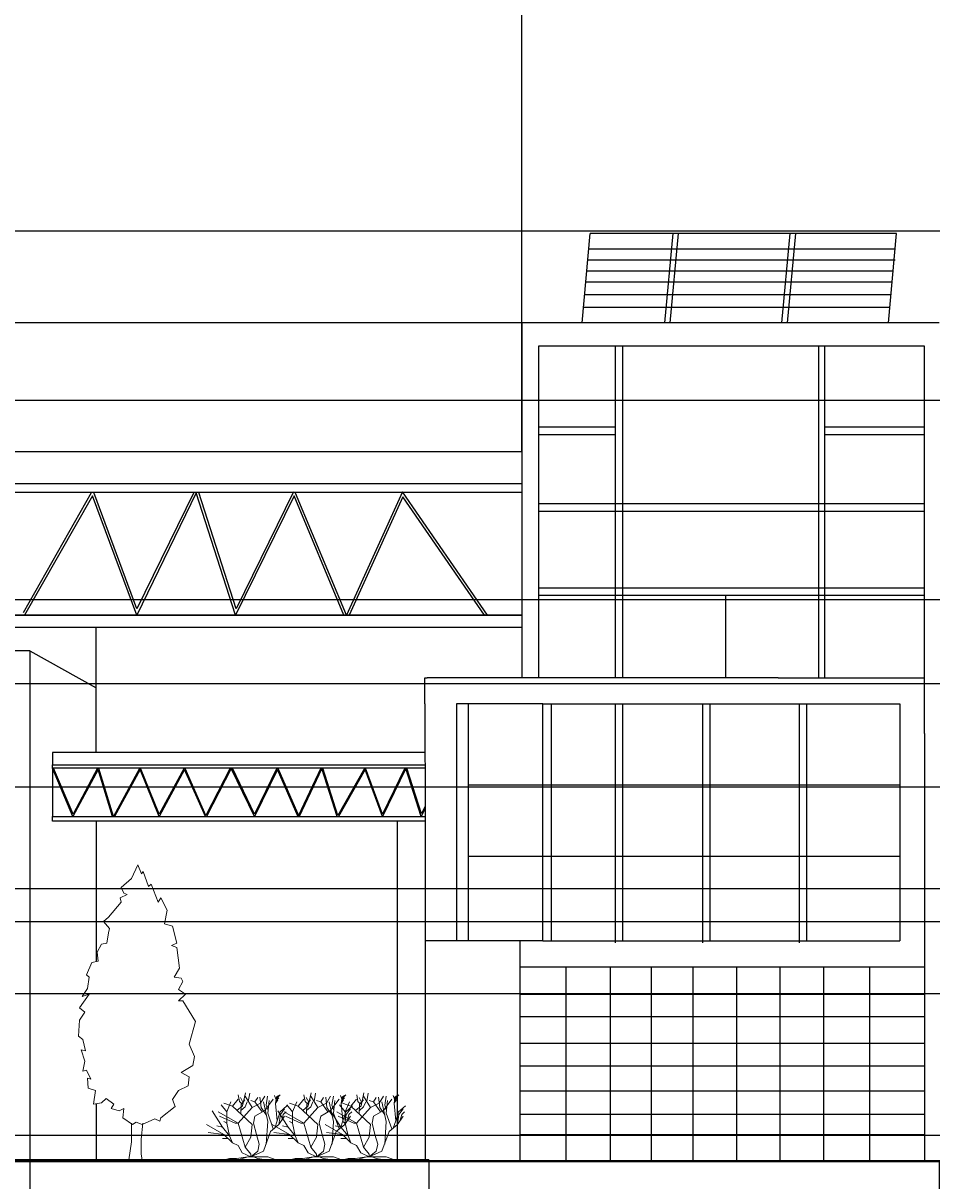
# Model space of a CAD drawing. Units: inches. Extents: x -32109 to 33221, y -19197 to 7608.
# Tile 11 of 25: x -9406 to -5707, y -2204 to 2510. Entities that reach past the tile are written whole.
import ezdxf

# ---------------------------------------------------------------- set-up
doc = ezdxf.new("R2010")
doc.units = ezdxf.units.IN
doc.header["$MEASUREMENT"] = 0
for name, color, linetype, lineweight in [('A-ANNO-DIMS', 2, 'Continuous', 18), ('A-ELEV', 7, 'Continuous', 25), ('L-PLNT', 3, 'Continuous', 13)]:
    doc.layers.add(name, color=color, linetype=linetype, lineweight=lineweight)
doc.styles.get("Standard").update_dxf_attribs({"font": 'arial.ttf'})
doc.dimstyles.get("Standard").update_dxf_attribs({"dimtxt": 0.18, "dimasz": 0.18, "dimexe": 0.18, "dimexo": 0.0625, "dimgap": 0.09, "dimtad": 0, "dimtih": 1, "dimtoh": 1, "dimdec": 4, "dimzin": 0, "dimdsep": 46, "dimtxsty": 'Standard', "dimcen": 0.09, "dimadec": 0, "dimazin": 0, "dimtfac": 1, "dimtdec": 4, "dimtofl": 0, "dimtmove": 0, "dimatfit": 3, "dimfxl": 1, "dimtolj": 1, "dimtzin": 0, "dimarcsym": 0})

# ---------------------------------------------------------------- blocks, each defined once
blk = doc.blocks.new('*U2')
blk.add_lwpolyline([(-2.754, 191.699), (-6.78, 182.851), (-13.682, 176.953), (-11.956, 173.266), (-9.656, 172.529), (-14.257, 170.317), (-13.682, 167.368), (-21.733, 157.783), (-25.184, 154.834), (-21.158, 150.41), (-21.733, 147.461), (-22.884, 140.825), (-26.334, 140.087), (-29.21, 134.926), (-28.635, 129.028), (-32.661, 128.291), (-36.111, 120.18), (-34.386, 118.706), (-35.536, 111.333), (-38.987, 106.171), (-34.386, 107.646), (-40.712, 98.798), (-37.261, 95.849), (-40.712, 90.688), (-41.287, 80.366), (-38.412, 78.154), (-36.686, 70.781), (-39.562, 71.518), (-37.261, 64.145), (-38.412, 57.509), (-36.111, 58.247), (-33.236, 52.348), (-35.536, 53.086), (-34.961, 46.45), (-30.36, 44.975), (-31.51, 36.128), (-26.334, 36.865), (-23.459, 39.814), (-18.283, 36.128), (-20.008, 33.178), (-14.832, 31.704), (-11.956, 33.178), (-12.531, 27.28), (-6.205, 22.856), (-3.905, 24.331), (0.121, 22.856), (8.173, 26.543), (11.624, 25.068), (12.199, 27.28), (21.4, 34.653), (19.675, 39.077), (23.701, 44.975), (30.027, 47.924), (30.602, 53.823), (25.426, 56.772), (32.903, 61.196), (34.053, 67.094), (30.602, 75.205), (34.628, 89.951), (26.576, 103.222), (23.701, 103.222), (28.302, 107.646), (23.701, 110.595), (26.576, 115.756), (25.426, 117.968), (20.825, 118.706), (24.276, 124.604), (22.551, 137.876), (19.1, 139.35), (22.551, 140.825), (19.675, 151.884), (14.499, 153.359), (16.224, 162.207), (12.199, 170.317), (10.473, 167.368), (5.872, 179.165), (4.147, 177.69), (0.696, 187.275), (-0.454, 185.8)], close=True)
for points in [[(-6.813, 23.669), (-6.813, 11.669), (-8.627, 0)], [(0.387, 23.669), (-0.576, 13.271), (-0.576, 3.686), (0, 0)]]:
    blk.add_lwpolyline(points)
blk = doc.blocks.new('*U3')
for p, q in [((-16.8, 16.32), (-15.36, 19.68)), ((-14.88, 18.24), (-12.96, 20.64)), ((-12.471, 19.775), (-12.898, 22.044)), ((-11.677, 19.071), (-12.471, 19.775)), ((-11.28, 19.619), (-12.104, 21.184)), ((-11.921, 18.836), (-10.64, 20.401)), ((-11.433, 18.289), (-10.457, 22.749)), ((-10.579, 18.054), (-9.846, 19.697)), ((-8.16, 17.76), (-10.56, 21.6)), ((-9.48, 19.775), (-8.992, 22.592)), ((-7.2, 19.68), (-8.64, 20.16)), ((-7.2, 19.68), (-6.24, 21.12)), ((-4.8, 16.32), (-7.2, 19.68)), ((-5.086, 17.741), (-5.513, 21.34)), ((-5.28, 19.2), (-3.84, 21.6)), ((-2.88, 12.96), (-4.32, 19.68)), ((-3.84, 16.8), (-0.96, 20.64)), ((-3.377, 18.602), (-2.888, 21.575)), ((-2.88, 15.84), (-2.4, 20.16)), ((-0.508, 21.888), (-0.081, 20.558)), ((-0.203, 19.149), (0.102, 21.34)), ((-0.142, 19.384), (0.59, 20.401)), ((-0.02, 20.01), (0.896, 21.105)), ((0.041, 20.714), (1.384, 22.044)), ((0.102, 21.34), (0.835, 21.888)), ((-18.24, 11.04), (-21.755, 16.655)), ((-12.96, 12.48), (-19.68, 16.32)), ((-16.8, 16.32), (-18.72, 18.72)), ((-14.88, 18.24), (-17.76, 19.2)), ((-16.8, 12.48), (-16.8, 16.32)), ((-8.16, 12), (-14.88, 18.24)), ((-13.325, 16.724), (-11.433, 18.289)), ((-12.96, 12.48), (-8.16, 17.76)), ((-12.043, 15.628), (-11.921, 18.836)), ((-11.982, 16.802), (-10.579, 18.054)), ((-8.16, 17.76), (-5.28, 19.2)), ((-7.2, 14.88), (-3.84, 16.8)), ((-3.377, 15.315), (-5.086, 17.819)), ((-2.766, 16.802), (-3.377, 18.602)), ((-0.96, 10.56), (-2.88, 15.84)), ((0.346, 13.203), (-0.203, 19.149)), ((0.346, 13.203), (1.323, 16.254)), ((1.323, 16.254), (3.642, 18.289)), ((1.44, 15.36), (2.88, 17.28)), ((2.4, 15.36), (3.36, 16.32)), ((-17.76, 8.64), (-23.663, 11.961)), ((-13.92, 12.48), (-19.2, 14.88)), ((-16.8, 12.48), (-17.76, 12.96)), ((-15.84, 8.16), (-16.8, 12.48)), ((-12.96, 12.48), (-13.92, 12.48)), ((-10.56, 4.32), (-12.96, 12.48)), ((-8.64, 7.68), (-8.16, 12)), ((-7.68, 12.48), (-7.2, 14.88)), ((-6.72, 8.64), (-7.68, 12.48)), ((-3.36, 5.28), (-2.88, 12.96)), ((-1.92, 9.6), (0.96, 12)), ((-0.48, 10.8), (0.346, 13.203)), ((0.96, 12), (1.44, 15.36)), ((0.96, 12), (2.88, 14.88)), ((1.92, 13.44), (2.4, 15.36)), ((-17.76, 8.64), (-23.128, 9.222)), ((-18.24, 11.04), (-20.16, 11.52)), ((-15.84, 8.16), (-18.24, 11.04)), ((-14.88, 5.76), (-17.76, 8.64)), ((-14.88, 5.76), (-15.84, 8.16)), ((-5.76, 5.28), (-6.72, 8.64)), ((-4.32, 2.88), (-1.92, 9.6)), ((-16.32, 7.2), (-18.24, 7.2)), ((-12.96, 4.8), (-14.88, 5.76)), ((-11.52, 2.4), (-12.96, 4.8)), ((-10.56, 4.32), (-8.64, 7.68)), ((-8.64, 1.92), (-10.56, 4.32)), ((-6.24, 2.88), (-5.76, 5.28)), ((-15.84, 0.48), (-17.76, 0)), ((-13.44, 0.48), (-15.84, 0.48)), ((-9.6, 0.96), (-13.44, 0.48)), ((-9.6, 0.96), (-12.96, 0)), ((-8.64, 0.96), (-11.52, 2.4)), ((-9.6, 0.96), (-7.68, 0.96)), ((-8.64, 0.96), (-4.32, 2.88)), ((-8.64, 0.96), (-6.24, 2.88)), ((-8.64, 0.96), (-8.64, 1.92)), ((-8.64, 0.96), (-2.88, 0.96)), ((-7.68, 0.96), (-6.24, 0.48)), ((-6.24, 0.48), (-3.36, 0)), ((-2.88, 0.96), (0, 0))]:
    blk.add_line(p, q)
blk = doc.blocks.new('*D10')
at = {"layer": 'A-ANNO-DIMS', "color": 0, "lineweight": -2, "transparency": 16777216}
for p, q in [((-18512.6, -110.2), (-18512.6, 5772)), ((-18512.5, 5771.8), (-202.1, 5771.8)), ((18109.1, 5771.8), (-201.2, 5771.8)), ((18109.3, -101.5), (18109.3, 5772))]:
    blk.add_line(p, q, dxfattribs=at)
at = {"layer": 'A-ANNO-DIMS', "color": 0, "transparency": 16777216}
for points in [[(-18512.5, 5771.9), (-18512.5, 5771.8), (-18512.6, 5771.8)], [(18109.1, 5771.9), (18109.1, 5771.8), (18109.3, 5771.8)]]:
    blk.add_solid(points, dxfattribs=at)
at = {"layer": 'Defpoints', "color": 0, "transparency": 16777216}
for p in [(18109.3, 5771.8), (-18512.6, -110.2), (18109.3, -101.6)]:
    blk.add_point(p, dxfattribs=at)
at = {"layer": 'A-ANNO-DIMS', "color": 0, "transparency": 16777216, "insert": (-201.7, 5771.8), "char_height": 0.18, "attachment_point": 5}
blk.add_mtext('\\A1;36622', dxfattribs=at)
blk = doc.blocks.new('*D11')
at = {"layer": 'A-ANNO-DIMS', "color": 0, "lineweight": -2, "transparency": 16777216}
for p, q in [((14509.6, 1705.2), (25710.6, 1705.2)), ((25710.5, 1705), (25710.5, -209.6)), ((25710.5, -2124.6), (25710.5, -210)), ((-18512.6, -2124.8), (25710.6, -2124.8))]:
    blk.add_line(p, q, dxfattribs=at)
at = {"layer": 'A-ANNO-DIMS', "color": 0, "transparency": 16777216}
for points in [[(25710.4, 1705), (25710.5, 1705), (25710.5, 1705.2)], [(25710.4, -2124.6), (25710.5, -2124.6), (25710.5, -2124.8)]]:
    blk.add_solid(points, dxfattribs=at)
at = {"layer": 'Defpoints', "color": 0, "transparency": 16777216}
for p in [(14509.6, 1705.2), (-18512.6, -2124.8), (25710.5, -2124.8)]:
    blk.add_point(p, dxfattribs=at)
at = {"layer": 'A-ANNO-DIMS', "color": 0, "transparency": 16777216, "insert": (25710.5, -209.8), "char_height": 0.18, "attachment_point": 5}
blk.add_mtext('\\A1;3830', dxfattribs=at)
blk = doc.blocks.new('*D21')
at = {"layer": 'A-ANNO-DIMS', "color": 0, "lineweight": -2, "transparency": 16777216}
for p, q in [((-5532.2, -1149.2), (-24362, -1149.2)), ((-24361.8, -1149.4), (-24361.8, -1636.8)), ((-24361.8, -2124.6), (-24361.8, -1637.2)), ((-5677.1, -2124.8), (-24362, -2124.8))]:
    blk.add_line(p, q, dxfattribs=at)
at = {"layer": 'A-ANNO-DIMS', "color": 0, "transparency": 16777216}
for points in [[(-24361.8, -1149.4), (-24361.8, -1149.4), (-24361.8, -1149.2)], [(-24361.8, -2124.6), (-24361.8, -2124.6), (-24361.8, -2124.8)]]:
    blk.add_solid(points, dxfattribs=at)
at = {"layer": 'Defpoints', "color": 0, "transparency": 16777216}
for p in [(-24361.8, -1149.2), (-5532.1, -1149.2), (-5677.1, -2124.8)]:
    blk.add_point(p, dxfattribs=at)
at = {"layer": 'A-ANNO-DIMS', "color": 0, "transparency": 16777216, "insert": (-24361.8, -1637), "char_height": 0.18, "attachment_point": 5}
blk.add_mtext('\\A1;975.6', dxfattribs=at)
blk = doc.blocks.new('*D27')
at = {"layer": 'A-ANNO-DIMS', "color": 0, "lineweight": -2, "transparency": 16777216}
for p, q in [((-11787, -2124.9), (-11787, -5429.7)), ((-9378.4, -2124.9), (-9378.4, -5429.7)), ((-11786.8, -5429.6), (-10583.2, -5429.6)), ((-9378.6, -5429.6), (-10582.2, -5429.6))]:
    blk.add_line(p, q, dxfattribs=at)
at = {"layer": 'A-ANNO-DIMS', "color": 0, "transparency": 16777216}
for points in [[(-11786.8, -5429.5), (-11786.8, -5429.6), (-11787, -5429.6)], [(-9378.6, -5429.5), (-9378.6, -5429.6), (-9378.4, -5429.6)]]:
    blk.add_solid(points, dxfattribs=at)
at = {"layer": 'Defpoints', "color": 0, "transparency": 16777216}
for p in [(-11787, -2124.8), (-9378.4, -2124.8), (-9378.4, -5429.6)]:
    blk.add_point(p, dxfattribs=at)
at = {"layer": 'A-ANNO-DIMS', "color": 0, "transparency": 16777216, "insert": (-10582.7, -5429.6), "char_height": 0.18, "attachment_point": 5}
blk.add_mtext('\\A1;2408.6', dxfattribs=at)
blk = doc.blocks.new('*D28')
at = {"layer": 'A-ANNO-DIMS', "color": 0, "lineweight": -2, "transparency": 16777216}
for p, q in [((-7754.4, -2118.5), (-7754.4, -5429.7)), ((-9378.4, -2124.9), (-9378.4, -5429.7)), ((-9378.2, -5429.6), (-8566.7, -5429.6)), ((-7754.6, -5429.6), (-8566, -5429.6))]:
    blk.add_line(p, q, dxfattribs=at)
at = {"layer": 'A-ANNO-DIMS', "color": 0, "transparency": 16777216}
for points in [[(-9378.2, -5429.5), (-9378.2, -5429.6), (-9378.4, -5429.6)], [(-7754.6, -5429.5), (-7754.6, -5429.6), (-7754.4, -5429.6)]]:
    blk.add_solid(points, dxfattribs=at)
at = {"layer": 'Defpoints', "color": 0, "transparency": 16777216}
for p in [(-7754.4, -2118.4), (-9378.4, -2124.8), (-7754.4, -5429.6)]:
    blk.add_point(p, dxfattribs=at)
at = {"layer": 'A-ANNO-DIMS', "color": 0, "transparency": 16777216, "insert": (-8566.4, -5429.6), "char_height": 0.18, "attachment_point": 5}
blk.add_mtext('\\A1;1624', dxfattribs=at)
blk = doc.blocks.new('*D29')
at = {"layer": 'A-ANNO-DIMS', "color": 0, "lineweight": -2, "transparency": 16777216}
for p, q in [((-7754.4, -2118.5), (-7754.4, -5429.7)), ((-5677.1, -2124.9), (-5677.1, -5429.7)), ((-7754.2, -5429.6), (-6716.2, -5429.6)), ((-5677.3, -5429.6), (-6715.3, -5429.6))]:
    blk.add_line(p, q, dxfattribs=at)
at = {"layer": 'A-ANNO-DIMS', "color": 0, "transparency": 16777216}
for points in [[(-7754.2, -5429.5), (-7754.2, -5429.6), (-7754.4, -5429.6)], [(-5677.3, -5429.5), (-5677.3, -5429.6), (-5677.1, -5429.6)]]:
    blk.add_solid(points, dxfattribs=at)
at = {"layer": 'Defpoints', "color": 0, "transparency": 16777216}
for p in [(-7754.4, -2118.4), (-5677.1, -2124.8), (-5677.1, -5429.6)]:
    blk.add_point(p, dxfattribs=at)
at = {"layer": 'A-ANNO-DIMS', "color": 0, "transparency": 16777216, "insert": (-6715.7, -5429.6), "char_height": 0.18, "attachment_point": 5}
blk.add_mtext('\\A1;2077.3', dxfattribs=at)
blk = doc.blocks.new('*D39')
at = {"layer": 'A-ANNO-DIMS', "color": 0, "lineweight": -2, "transparency": 16777216}
for p, q in [((-7375.9, 1290), (-24362, 1290)), ((-24361.8, 1289.8), (-24361.8, -414)), ((-24361.8, -2118.3), (-24361.8, -414.4)), ((-7754.5, -2118.4), (-24362, -2118.4))]:
    blk.add_line(p, q, dxfattribs=at)
at = {"layer": 'A-ANNO-DIMS', "color": 0, "transparency": 16777216}
for points in [[(-24361.8, 1289.8), (-24361.8, 1289.8), (-24361.8, 1290)], [(-24361.8, -2118.3), (-24361.8, -2118.3), (-24361.8, -2118.4)]]:
    blk.add_solid(points, dxfattribs=at)
at = {"layer": 'Defpoints', "color": 0, "transparency": 16777216}
for p in [(-7375.9, 1290), (-24361.8, -2118.4), (-7754.4, -2118.4)]:
    blk.add_point(p, dxfattribs=at)
at = {"layer": 'A-ANNO-DIMS', "color": 0, "transparency": 16777216, "insert": (-24361.8, -414.2), "char_height": 0.18, "attachment_point": 5}
blk.add_mtext('\\A1;3408.5', dxfattribs=at)
blk = doc.blocks.new('*D40')
at = {"layer": 'A-ANNO-DIMS', "color": 0, "lineweight": -2, "transparency": 16777216}
for p, q in [((-5445.1, 973), (-24362, 973)), ((-24361.8, 972.8), (-24361.8, -575.7)), ((-24361.8, -2124.6), (-24361.8, -576.1)), ((-5677.1, -2124.8), (-24362, -2124.8))]:
    blk.add_line(p, q, dxfattribs=at)
at = {"layer": 'A-ANNO-DIMS', "color": 0, "transparency": 16777216}
for points in [[(-24361.8, 972.8), (-24361.8, 972.8), (-24361.8, 973)], [(-24361.8, -2124.6), (-24361.8, -2124.6), (-24361.8, -2124.8)]]:
    blk.add_solid(points, dxfattribs=at)
at = {"layer": 'Defpoints', "color": 0, "transparency": 16777216}
for p in [(-5445, 973), (-24361.8, -2124.8), (-5677.1, -2124.8)]:
    blk.add_point(p, dxfattribs=at)
at = {"layer": 'A-ANNO-DIMS', "color": 0, "transparency": 16777216, "insert": (-24361.8, -575.9), "char_height": 0.18, "attachment_point": 5}
blk.add_mtext('\\A1;3098', dxfattribs=at)
blk = doc.blocks.new('*D41')
at = {"layer": 'A-ANNO-DIMS', "color": 0, "lineweight": -2, "transparency": 16777216}
for p, q in [((-651, 162.2), (-24362, 162.2)), ((-24361.8, 162), (-24361.8, -981.1)), ((-24361.8, -2124.6), (-24361.8, -981.5)), ((-651, -2124.8), (-24362, -2124.8))]:
    blk.add_line(p, q, dxfattribs=at)
at = {"layer": 'A-ANNO-DIMS', "color": 0, "transparency": 16777216}
for points in [[(-24361.8, 162), (-24361.8, 162), (-24361.8, 162.2)], [(-24361.8, -2124.6), (-24361.8, -2124.6), (-24361.8, -2124.8)]]:
    blk.add_solid(points, dxfattribs=at)
at = {"layer": 'Defpoints', "color": 0, "transparency": 16777216}
for p in [(-651, 162.2), (-24361.8, -2124.8), (-651, -2124.8)]:
    blk.add_point(p, dxfattribs=at)
at = {"layer": 'A-ANNO-DIMS', "color": 0, "transparency": 16777216, "insert": (-24361.8, -981.3), "char_height": 0.18, "attachment_point": 5}
blk.add_mtext('\\A1;2287', dxfattribs=at)
blk = doc.blocks.new('*D43')
at = {"layer": 'A-ANNO-DIMS', "color": 0, "lineweight": -2, "transparency": 16777216}
for p, q in [((-7375.9, 99.1), (-24362, 99.1)), ((-24361.8, 98.9), (-24361.8, -1009.5)), ((-24361.8, -2118.3), (-24361.8, -1009.8)), ((-7754.5, -2118.4), (-24362, -2118.4))]:
    blk.add_line(p, q, dxfattribs=at)
at = {"layer": 'A-ANNO-DIMS', "color": 0, "transparency": 16777216}
for points in [[(-24361.8, 98.9), (-24361.8, 98.9), (-24361.8, 99.1)], [(-24361.8, -2118.3), (-24361.8, -2118.3), (-24361.8, -2118.4)]]:
    blk.add_solid(points, dxfattribs=at)
at = {"layer": 'Defpoints', "color": 0, "transparency": 16777216}
for p in [(-7375.9, 99.1), (-24361.8, -2118.4), (-7754.4, -2118.4)]:
    blk.add_point(p, dxfattribs=at)
at = {"layer": 'A-ANNO-DIMS', "color": 0, "transparency": 16777216, "insert": (-24361.8, -1009.7), "char_height": 0.18, "attachment_point": 5}
blk.add_mtext('\\A1;2217.5', dxfattribs=at)
blk = doc.blocks.new('*D44')
at = {"layer": 'A-ANNO-DIMS', "color": 0, "lineweight": -2, "transparency": 16777216}
for p, q in [((-12501.4, 764.2), (-12501.4, 5772)), ((-12501.2, 5771.8), (-9939, 5771.8)), ((-7376.1, 5771.8), (-9938.3, 5771.8)), ((-7375.9, 764.2), (-7375.9, 5772))]:
    blk.add_line(p, q, dxfattribs=at)
at = {"layer": 'A-ANNO-DIMS', "color": 0, "transparency": 16777216}
for points in [[(-12501.2, 5771.9), (-12501.2, 5771.8), (-12501.4, 5771.8)], [(-7376.1, 5771.9), (-7376.1, 5771.8), (-7375.9, 5771.8)]]:
    blk.add_solid(points, dxfattribs=at)
at = {"layer": 'Defpoints', "color": 0, "transparency": 16777216}
for p in [(-7375.9, 5771.8), (-12501.4, 764.2), (-7375.9, 764.2)]:
    blk.add_point(p, dxfattribs=at)
at = {"layer": 'A-ANNO-DIMS', "color": 0, "transparency": 16777216, "insert": (-9938.6, 5771.8), "char_height": 0.18, "attachment_point": 5}
blk.add_mtext('\\A1;5125', dxfattribs=at)
blk = doc.blocks.new('*D53')
at = {"layer": 'A-ANNO-DIMS', "color": 0, "lineweight": -2, "transparency": 16777216}
for p, q in [((-9508.3, -179.7), (25710.6, -179.7)), ((25710.5, -179.9), (25710.5, -389.7)), ((25710.5, -600), (25710.5, -390.1)), ((-9508.3, -600.2), (25710.6, -600.2))]:
    blk.add_line(p, q, dxfattribs=at)
at = {"layer": 'A-ANNO-DIMS', "color": 0, "transparency": 16777216}
for points in [[(25710.4, -179.9), (25710.5, -179.9), (25710.5, -179.7)], [(25710.4, -600), (25710.5, -600), (25710.5, -600.2)]]:
    blk.add_solid(points, dxfattribs=at)
at = {"layer": 'Defpoints', "color": 0, "transparency": 16777216}
for p in [(-9508.3, -179.7), (-9508.3, -600.2), (25710.5, -600.2)]:
    blk.add_point(p, dxfattribs=at)
at = {"layer": 'A-ANNO-DIMS', "color": 0, "transparency": 16777216, "insert": (25710.5, -389.9), "char_height": 0.18, "attachment_point": 5}
blk.add_mtext('\\A1;420.5', dxfattribs=at)
blk = doc.blocks.new('*D54')
at = {"layer": 'A-ANNO-DIMS', "color": 0, "lineweight": -2, "transparency": 16777216}
for p, q in [((-9508.3, -600.2), (25710.6, -600.2)), ((25710.5, -600.3), (25710.5, -806.8)), ((25710.5, -1013.7), (25710.5, -807.2)), ((-9508.3, -1013.9), (25710.6, -1013.9))]:
    blk.add_line(p, q, dxfattribs=at)
at = {"layer": 'A-ANNO-DIMS', "color": 0, "transparency": 16777216}
for points in [[(25710.4, -600.3), (25710.5, -600.3), (25710.5, -600.2)], [(25710.4, -1013.7), (25710.5, -1013.7), (25710.5, -1013.9)]]:
    blk.add_solid(points, dxfattribs=at)
at = {"layer": 'Defpoints', "color": 0, "transparency": 16777216}
for p in [(-9508.3, -600.2), (-9508.3, -1013.9), (25710.5, -1013.9)]:
    blk.add_point(p, dxfattribs=at)
at = {"layer": 'A-ANNO-DIMS', "color": 0, "transparency": 16777216, "insert": (25710.5, -807), "char_height": 0.18, "attachment_point": 5}
blk.add_mtext('\\A1;413.7', dxfattribs=at)
blk = doc.blocks.new('*D55')
at = {"layer": 'A-ANNO-DIMS', "color": 0, "lineweight": -2, "transparency": 16777216}
for p, q in [((-9508.3, -1013.9), (25710.6, -1013.9)), ((25710.5, -1014.1), (25710.5, -1227.7)), ((25710.5, -1441.6), (25710.5, -1228)), ((-9508.3, -1441.8), (25710.6, -1441.8))]:
    blk.add_line(p, q, dxfattribs=at)
at = {"layer": 'A-ANNO-DIMS', "color": 0, "transparency": 16777216}
for points in [[(25710.4, -1014.1), (25710.5, -1014.1), (25710.5, -1013.9)], [(25710.4, -1441.6), (25710.5, -1441.6), (25710.5, -1441.8)]]:
    blk.add_solid(points, dxfattribs=at)
at = {"layer": 'Defpoints', "color": 0, "transparency": 16777216}
for p in [(-9508.3, -1013.9), (-9508.3, -1441.8), (25710.5, -1441.8)]:
    blk.add_point(p, dxfattribs=at)
at = {"layer": 'A-ANNO-DIMS', "color": 0, "transparency": 16777216, "insert": (25710.5, -1227.9), "char_height": 0.18, "attachment_point": 5}
blk.add_mtext('\\A1;427.9', dxfattribs=at)
blk = doc.blocks.new('*D56')
at = {"layer": 'A-ANNO-DIMS', "color": 0, "lineweight": -2, "transparency": 16777216}
for p, q in [((-9508.3, -1441.8), (25710.6, -1441.8)), ((25710.5, -1442), (25710.5, -1730.1)), ((25710.5, -2018.6), (25710.5, -1730.5)), ((-9508.3, -2018.8), (25710.6, -2018.8))]:
    blk.add_line(p, q, dxfattribs=at)
at = {"layer": 'A-ANNO-DIMS', "color": 0, "transparency": 16777216}
for points in [[(25710.4, -1442), (25710.5, -1442), (25710.5, -1441.8)], [(25710.4, -2018.6), (25710.5, -2018.6), (25710.5, -2018.8)]]:
    blk.add_solid(points, dxfattribs=at)
at = {"layer": 'Defpoints', "color": 0, "transparency": 16777216}
for p in [(-9508.3, -1441.8), (-9508.3, -2018.8), (25710.5, -2018.8)]:
    blk.add_point(p, dxfattribs=at)
at = {"layer": 'A-ANNO-DIMS', "color": 0, "transparency": 16777216, "insert": (25710.5, -1730.3), "char_height": 0.18, "attachment_point": 5}
blk.add_mtext('\\A1;576.9', dxfattribs=at)
blk = doc.blocks.new('*D158')
at = {"layer": 'A-ANNO-DIMS', "color": 0, "lineweight": -2, "transparency": 16777216}
for p, q in [((5447.3, 1662.2), (-24362, 1662.2)), ((-24361.8, 1662), (-24361.8, -230.1)), ((-24361.8, -2122.6), (-24361.8, -230.5)), ((5279.2, -2122.7), (-24362, -2122.7))]:
    blk.add_line(p, q, dxfattribs=at)
at = {"layer": 'A-ANNO-DIMS', "color": 0, "transparency": 16777216}
for points in [[(-24361.8, 1662), (-24361.8, 1662), (-24361.8, 1662.2)], [(-24361.8, -2122.6), (-24361.8, -2122.6), (-24361.8, -2122.7)]]:
    blk.add_solid(points, dxfattribs=at)
at = {"layer": 'Defpoints', "color": 0, "transparency": 16777216}
for p in [(5447.3, 1662.2), (-24361.8, -2122.7), (5279.3, -2122.7)]:
    blk.add_point(p, dxfattribs=at)
at = {"layer": 'A-ANNO-DIMS', "color": 0, "transparency": 16777216, "insert": (-24361.8, -230.3), "char_height": 0.18, "attachment_point": 5}
blk.add_mtext('\\A1;3784.9', dxfattribs=at)

msp = doc.modelspace()

# ---------------------------------------------------------------- linework, layer by layer
at = {"layer": 'A-ELEV'}
for p, q in [((-7131.208, 1290.029), (-7097.87, 1653.528)), ((-5850.659, 1653.528), (-7097.87, 1653.528)), ((-6793.683, 1290.029), (-6760.345, 1653.528)), ((-6771.676, 1290.029), (-6738.339, 1653.528)), ((-6317.542, 1290.029), (-6284.204, 1653.528)), ((-6294.041, 1290.029), (-6260.703, 1653.528)), ((-6294.041, 1290.029), (-6260.703, 1653.528)), ((-5883.996, 1290.029), (-5850.659, 1653.528)), ((-5856.587, 1588.89), (-7103.798, 1588.89)), ((-5856.587, 1544.135), (-7107.903, 1544.135)), ((-5864.796, 1499.379), (-7112.007, 1499.379)), ((-5868.901, 1454.624), (-7116.112, 1454.624)), ((-5873.592, 1403.475), (-7120.803, 1403.475)), ((-5878.283, 1352.326), (-7125.494, 1352.326)), ((-5677.079, 1290.029), (-7375.878, 1290.029)), ((-7375.878, 1290.029), (-7375.878, -156.541)), ((-5737.208, 1195.158), (-7308.584, 1195.158)), ((-7308.584, 1195.158), (-7308.584, -156.541)), ((-5737.208, 1195.158), (-7308.584, 1195.158)), ((-6995.828, 1195.158), (-6995.828, -156.541)), ((-6965.748, 1195.158), (-6965.748, -156.541)), ((-6169.106, 1195.158), (-6169.106, -156.541)), ((-6144.383, 1195.158), (-6144.383, -156.541)), ((-5737.208, -382.433), (-5737.208, 1195.158)), ((-6995.828, 864.24), (-7308.584, 864.24)), ((-5737.208, 864.24), (-6144.383, 864.24)), ((-6995.828, 833.746), (-7308.584, 833.746)), ((-5737.208, 833.746), (-6144.383, 833.746)), ((-7375.878, 764.187), (-12501.359, 764.187)), ((-12501.359, 635.262), (-7375.878, 635.262)), ((-7375.878, 598.924), (-12501.359, 598.924)), ((-9128.716, 597.893), (-9406.073, 109.271)), ((-9124.177, 585.632), (-9400.345, 99.103)), ((-8944.003, 98.938), (-9124.177, 585.632)), ((-8942.755, 124.371), (-9118.434, 598.924)), ((-8701.313, 597.995), (-8944.003, 98.938)), ((-8711.981, 598.924), (-8942.755, 124.371)), ((-8541.424, 98.938), (-8701.313, 597.995)), ((-8539.472, 125.622), (-8691.11, 598.924)), ((-8303.167, 584.622), (-8541.424, 98.938)), ((-8306.284, 600.973), (-8539.472, 125.622)), ((-8101.206, 99.103), (-8303.167, 584.622)), ((-8090.306, 98.938), (-8297.306, 596.569)), ((-7861.893, 600.847), (-8090.306, 98.938)), ((-7860.103, 580.636), (-8079.244, 99.103)), ((-7515.914, 99.103), (-7861.893, 600.847)), ((-7528.061, 99.103), (-7860.103, 580.636)), ((-5737.208, 552.318), (-7308.584, 552.318)), ((-5737.208, 521.824), (-7308.584, 521.824)), ((-5737.208, 209.629), (-7308.584, 209.629)), ((-5737.208, 179.136), (-7308.584, 179.136)), ((-6547.316, 179.136), (-6547.316, -156.541)), ((-12501.359, 99.103), (-7375.878, 99.103)), ((-6995.828, 117.191), (-6995.828, -156.541)), ((-7375.878, 49.157), (-12501.359, 49.157)), ((-9108.468, -196.107), (-9108.468, 48.673)), ((-9378.383, -45.544), (-11787.012, -45.544)), ((-9378.383, -45.544), (-9378.383, -740.123)), ((-9378.383, -45.544), (-9108.468, -196.107)), ((-7770.777, -261.89), (-7770.777, -156.541)), ((-7770.777, -156.541), (-7761.914, -156.541)), ((-7308.584, -156.541), (-7761.914, -156.541)), ((-6332.168, -156.541), (-7308.584, -156.541)), ((-6332.168, -156.541), (-5737.208, -156.541)), ((-9108.468, -459.533), (-9108.468, -196.107)), ((-7770.777, -261.89), (-7769.33, -740.123)), ((-7290.87, -261.89), (-7641.787, -261.89)), ((-7641.787, -261.89), (-7641.787, -1226.716)), ((-7593.599, -1226.716), (-7593.599, -261.89)), ((-7290.87, -1226.716), (-7290.87, -261.89)), ((-7290.87, -261.89), (-5837.049, -261.89)), ((-7255.048, -1226.716), (-7255.048, -261.89)), ((-6995.828, -261.89), (-6995.828, -1234.508)), ((-6965.748, -261.89), (-6965.748, -1226.716)), ((-6640.709, -261.89), (-6640.709, -1234.508)), ((-6610.629, -261.89), (-6610.629, -1226.716)), ((-6247.812, -261.89), (-6247.812, -1234.508)), ((-6217.732, -261.89), (-6217.732, -1226.716)), ((-5837.049, -261.89), (-5837.049, -1226.716)), ((-5737.208, -382.433), (-5737.208, -2124.791)), ((-7770.179, -459.533), (-9286.545, -459.533)), ((-9286.545, -459.533), (-9286.545, -510.125)), ((-9286.545, -510.125), (-7770.026, -510.125)), ((-9286.545, -524.385), (-9286.545, -510.125)), ((-9203.398, -720.66), (-9286.545, -524.317)), ((-9286.545, -524.385), (-9286.545, -720.523)), ((-7769.983, -524.385), (-9286.545, -524.385)), ((-9202.986, -711.569), (-9282.255, -524.385)), ((-9101.181, -529.536), (-9203.398, -720.66)), ((-9102.876, -524.385), (-9202.986, -711.569)), ((-9042.7, -720.523), (-9101.181, -529.536)), ((-9038.56, -720.64), (-9098.571, -524.656)), ((-8932.077, -524.685), (-9038.56, -720.64)), ((-8930.167, -529.387), (-9034.03, -720.523)), ((-8852.45, -720.674), (-8930.167, -529.387)), ((-8851.946, -711.49), (-8927.963, -524.385)), ((-8748.884, -529.118), (-8852.45, -720.674)), ((-8750.786, -524.385), (-8851.946, -711.49)), ((-8664.505, -720.523), (-8748.884, -529.118)), ((-8662.184, -716.059), (-8746.522, -524.749)), ((-8562.94, -524.385), (-8662.184, -716.059)), ((-8558.693, -524.718), (-8660.152, -720.669)), ((-8463.896, -720.648), (-8558.693, -524.718)), ((-8463.886, -711.657), (-8554.495, -524.385)), ((-8370.837, -529.309), (-8463.896, -720.648)), ((-8372.806, -524.385), (-8463.886, -711.657)), ((-8286.405, -722.199), (-8370.837, -529.309)), ((-8282.81, -720.625), (-8368.582, -524.674)), ((-8193.888, -524.385), (-8286.354, -718.941)), ((-8189.668, -524.648), (-8282.81, -720.625)), ((-8127.635, -720.523), (-8189.668, -524.648)), ((-8124.782, -716.533), (-8185.635, -524.385)), ((-8015.943, -524.79), (-8124.782, -716.533)), ((-8014.162, -529.601), (-8122.535, -720.523)), ((-7943.458, -720.588), (-8014.162, -529.601)), ((-7942.969, -710.608), (-8011.908, -524.385)), ((-7848.223, -524.75), (-7943.458, -720.588)), ((-7852.409, -524.385), (-7942.969, -710.608)), ((-7785.48, -720.588), (-7848.223, -524.75)), ((-7784.714, -710.117), (-7844.219, -524.385)), ((-7593.599, -591.207), (-5837.049, -591.207)), ((-7769.488, -687.99), (-7785.48, -720.588)), ((-7769.515, -679.134), (-7784.714, -710.117)), ((-9378.383, -740.123), (-9378.383, -2124.791)), ((-9286.545, -720.523), (-7769.39, -720.523)), ((-9286.545, -740.123), (-9286.545, -720.523)), ((-7769.33, -740.123), (-9286.545, -740.123)), ((-9108.468, -740.123), (-9108.468, -1311.302)), ((-8660.152, -720.669), (-8660.216, -720.523)), ((-7883.381, -740.123), (-7883.381, -2124.791)), ((-7769.33, -740.123), (-7769.33, -2124.791)), ((-7593.599, -881.903), (-5837.049, -881.903)), ((-7641.787, -1226.716), (-7769.33, -1226.716)), ((-7290.87, -1226.716), (-7641.787, -1226.716)), ((-7383.301, -1332.578), (-7383.301, -1226.716)), ((-7290.87, -1226.716), (-5837.049, -1226.716)), ((-7383.053, -1332.578), (-7383.301, -1332.578)), ((-7383.301, -2124.791), (-7383.301, -1332.578)), ((-7383.053, -1332.578), (-7290.87, -1332.578)), ((-7290.87, -1332.578), (-5837.049, -1332.578)), ((-7196.048, -2124.791), (-7196.048, -1332.578)), ((-7015.605, -2124.791), (-7015.605, -1332.578)), ((-6848.78, -2124.791), (-6848.78, -1332.578)), ((-6678.55, -2124.791), (-6678.55, -1332.578)), ((-6501.512, -2124.791), (-6501.512, -1332.578)), ((-6324.473, -2124.791), (-6324.473, -1332.578)), ((-6147.434, -2124.791), (-6147.434, -1332.578)), ((-5960.182, -2124.791), (-5960.182, -1332.578)), ((-5837.049, -1332.578), (-5737.208, -1332.578)), ((-7383.301, -1443.588), (-5737.208, -1443.588)), ((-7383.301, -1534.981), (-5737.208, -1534.981)), ((-7383.301, -1644.219), (-5737.208, -1644.219)), ((-7383.301, -1736.033), (-5737.208, -1736.033)), ((-7383.301, -1838.048), (-5737.208, -1838.048)), ((-9108.468, -1890.251), (-9108.468, -2124.791)), ((-7383.301, -1933.263), (-5737.208, -1933.263)), ((-7383.301, -2014.875), (-5737.208, -2014.875)), ((-18512.647, -2124.791), (1683.588, -2124.791)), ((-3437.624, -2124.791), (-10277.124, -2124.791)), ((-7769.33, -2124.791), (-5737.208, -2124.791)), ((-5677.079, -2124.791), (-5737.208, -2124.791))]:
    msp.add_line(p, q, dxfattribs=at)

# ---------------------------------------------------------------- block references
at = {"layer": 'L-PLNT'}
for name, p, xscale, yscale, zscale in [('*U2', (-8921.928, -2118.049), 6.26271834465589, 6.26271834465589, 6.26271834465589), ('*U3', (-8376.233, -2118.431), 11.97885450539613, 11.97885450539613, 11.97885450539613), ('*U3', (-8108.535, -2118.431), 11.97885450539613, 11.97885450539613, 11.97885450539613), ('*U3', (-7893.846, -2118.431), 11.97885450539613, 11.97885450539613, 11.97885450539613)]:
    msp.add_blockref(name, p, dxfattribs=dict(at, xscale=xscale, yscale=yscale, zscale=zscale))

# ---------------------------------------------------------------- dimensions: what is measured, and where the dimension line sits
at = {"layer": 'A-ANNO-DIMS'}
for base, p1, p2, override, picture, middle in [((18109.317, 5771.835), (-18512.647, -110.242), (18109.317, -101.6), {"dimdec": 0, "dimlfac": 1, "dimrnd": 0, "dimzin": 0, "dimdsep": 46, "dimlunit": 2}, '*D10', (-201.665, 5771.835)), ((-7375.878, 5771.835), (-12501.359, 764.187), (-7375.878, 764.187), {"dimdec": 0, "dimlfac": 1, "dimrnd": 0, "dimzin": 0, "dimdsep": 46, "dimlunit": 2}, '*D44', (-9938.618, 5771.835)), ((-7754.412, -5429.555), (-9378.383, -2124.791), (-7754.412, -2118.431), {"dimdec": 0, "dimlfac": 1, "dimrnd": 0, "dimzin": 0, "dimdsep": 46, "dimlunit": 2}, '*D28', (-8566.398, -5429.555)), ((-5677.079, -5429.555), (-7754.412, -2118.431), (-5677.079, -2124.791), {"dimdec": 1, "dimlfac": 1, "dimrnd": 0, "dimzin": 0, "dimdsep": 46, "dimlunit": 2}, '*D29', (-6715.746, -5429.555)), ((-9378.383, -5429.555), (-11787.012, -2124.791), (-9378.383, -2124.791), {"dimdec": 1, "dimlfac": 1, "dimrnd": 0, "dimzin": 0, "dimdsep": 46, "dimlunit": 2}, '*D27', (-10582.697, -5429.555))]:
    dim = msp.add_linear_dim(base=base, p1=p1, p2=p2, dimstyle='Standard', override=override, dxfattribs=at)
    dim.commit()
    dim.dimension.update_dxf_attribs({"geometry": picture, "text_midpoint": middle})
for base, p1, p2, override, picture, middle in [((25710.469, -2124.791), (14509.55, 1705.162), (-18512.647, -2124.791), {"dimdec": 0, "dimlfac": 1, "dimrnd": 0, "dimzin": 0, "dimdsep": 46, "dimlunit": 2}, '*D11', (25710.469, -209.814)), ((-24361.816, -2122.749), (5447.329, 1662.17), (5279.264, -2122.749), {"dimdec": 1, "dimlfac": 1, "dimrnd": 0, "dimzin": 0, "dimdsep": 46, "dimlunit": 2}, '*D158', (-24361.816, -230.29)), ((-24361.816, -2118.431), (-7375.878, 1290.029), (-7754.412, -2118.431), {"dimdec": 1, "dimlfac": 1, "dimrnd": 0, "dimzin": 0, "dimdsep": 46, "dimlunit": 2}, '*D39', (-24361.816, -414.201)), ((-24361.816, -2124.791), (-5445.024, 973.011), (-5677.079, -2124.791), {"dimdec": 0, "dimlfac": 1, "dimrnd": 0, "dimzin": 0, "dimdsep": 46, "dimlunit": 2}, '*D40', (-24361.816, -575.89)), ((-24361.816, -2124.791), (-650.959, 162.186), (-650.959, -2124.791), {"dimdec": 0, "dimlfac": 1, "dimrnd": 0, "dimzin": 0, "dimdsep": 46, "dimlunit": 2}, '*D41', (-24361.816, -981.302)), ((-24361.816, -2118.431), (-7375.878, 99.103), (-7754.412, -2118.431), {"dimdec": 1, "dimlfac": 1, "dimrnd": 0, "dimzin": 0, "dimdsep": 46, "dimlunit": 2}, '*D43', (-24361.816, -1009.664)), ((25710.469, -600.154), (-9508.333, -179.679), (-9508.333, -600.154), {"dimdec": 1, "dimlfac": 1, "dimrnd": 0, "dimzin": 0, "dimdsep": 46, "dimlunit": 2}, '*D53', (25710.469, -389.916)), ((25710.469, -1013.888), (-9508.333, -600.154), (-9508.333, -1013.888), {"dimdec": 1, "dimlfac": 1, "dimrnd": 0, "dimzin": 0, "dimdsep": 46, "dimlunit": 2}, '*D54', (25710.469, -807.021)), ((25710.469, -1441.815), (-9508.333, -1013.888), (-9508.333, -1441.815), {"dimdec": 1, "dimlfac": 1, "dimrnd": 0, "dimzin": 0, "dimdsep": 46, "dimlunit": 2}, '*D55', (25710.469, -1227.851)), ((-24361.816, -1149.23), (-5677.079, -2124.791), (-5532.101, -1149.23), {"dimdec": 1, "dimlfac": 1, "dimrnd": 0, "dimzin": 0, "dimdsep": 46, "dimlunit": 2}, '*D21', (-24361.816, -1637.01)), ((25710.469, -2018.754), (-9508.333, -1441.815), (-9508.333, -2018.754), {"dimdec": 1, "dimlfac": 1, "dimrnd": 0, "dimzin": 0, "dimdsep": 46, "dimlunit": 2}, '*D56', (25710.469, -1730.285))]:
    dim = msp.add_linear_dim(base=base, p1=p1, p2=p2, angle=90, dimstyle='Standard', override=override, dxfattribs=at)
    dim.commit()
    dim.dimension.update_dxf_attribs({"geometry": picture, "text_midpoint": middle})

doc.saveas('drawing.dxf')
